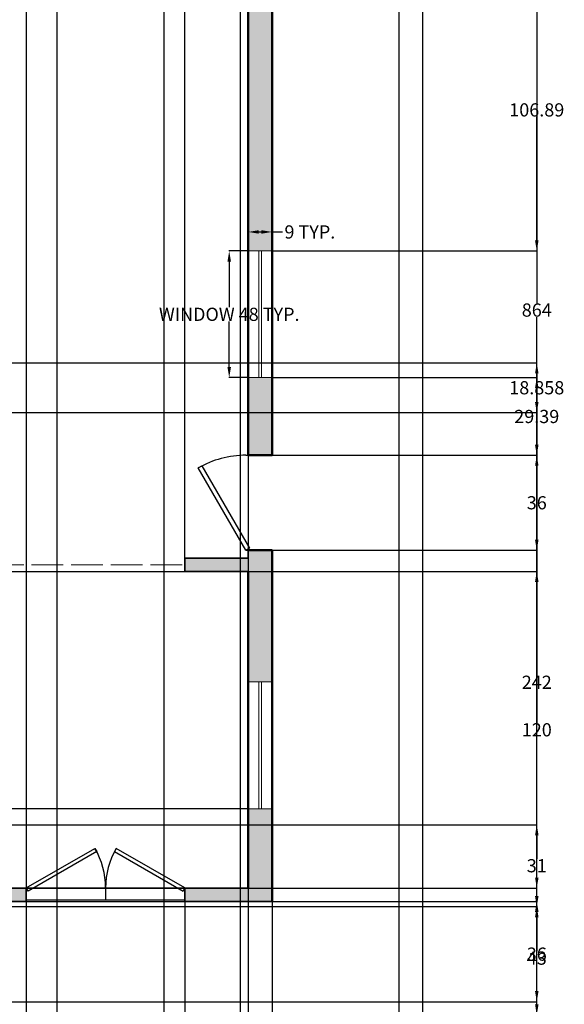
# Model space of a CAD drawing. Units: inches. Extents: x 882 to 1363, y 890 to 1847.
# Tile 6 of 9: x 1157 to 1363, y 1106 to 1479. Entities that reach past the tile are written whole.
import ezdxf

# ---------------------------------------------------------------- set-up
doc = ezdxf.new("R2010")
doc.units = ezdxf.units.IN
doc.header["$MEASUREMENT"] = 0
doc.linetypes.add('ACAD_ISO02W100', pattern=[15, 12, -3])
for name, color, linetype, lineweight in [('A-ANNO-DIMS', 2, 'Continuous', 18), ('A-WALL-OVHD', 7, 'ACAD_ISO02W100', 18), ('C-PROP', 7, 'Continuous', 25), ('doors', 3, 'Continuous', 25), ('inner wall', 50, 'Continuous', 35), ('outer wall', 40, 'Continuous', 50), ('windows', 226, 'Continuous', 18)]:
    doc.layers.add(name, color=color, linetype=linetype, lineweight=lineweight)
doc.layers.add('A-WALL-PATT', color=251, linetype='Continuous', lineweight=13, true_color=0x636466)
doc.styles.get("Standard").update_dxf_attribs({"font": 'arial.ttf'})
doc.dimstyles.get("Standard").update_dxf_attribs({"dimtxt": 5, "dimasz": 4, "dimexe": 0.18, "dimexo": 0.0625, "dimgap": 0.09, "dimtad": 0, "dimtih": 1, "dimtoh": 1, "dimdec": 1, "dimzin": 0, "dimdsep": 46, "dimlunit": 3, "dimtxsty": 'Standard', "dimcen": 0.09, "dimadec": 0, "dimazin": 0, "dimtfac": 1, "dimtdec": 1, "dimtofl": 0, "dimtmove": 0, "dimatfit": 3, "dimfxl": 1, "dimtolj": 1, "dimtzin": 0, "dimarcsym": 0})

# ---------------------------------------------------------------- blocks, each defined once
blk = doc.blocks.new('*U2')
for p, q in [((0, 0), (0, -6)), ((40, 0), (40, -6))]:
    blk.add_line(p, q)
blk.add_lwpolyline([(0, 0), (34.64, 20), (35.52, 18.48), (0.87, -1.52)], close=True)
blk.add_arc((0, 0), 40, 0, 30)
blk = doc.blocks.new('*U4')
for p, q in [((0, 0), (0, -6)), ((-40, 0), (-40, -6))]:
    blk.add_line(p, q)
blk.add_lwpolyline([(0, 0), (-34.64, 20), (-35.52, 18.48), (-0.88, -1.52)], close=True)
blk.add_arc((0, 0), 40, 150, 180)
blk = doc.blocks.new('WIN-48IN-9IN')
for p, q in [((4, 0), (4, 48)), ((5, 0), (5, 48))]:
    blk.add_line(p, q)
blk.add_lwpolyline([(0, 48), (9, 48), (9, 0), (0, 0)], close=True)
blk = doc.blocks.new('*D15')
at = {"layer": 'A-ANNO-DIMS', "color": 0, "lineweight": -2, "transparency": 16777216}
for p, q in [((1243.78, 1391.14), (1236.46, 1391.14)), ((1236.64, 1387.14), (1236.64, 1369.82)), ((1236.64, 1347.14), (1236.64, 1364.46)), ((1243.78, 1343.14), (1236.46, 1343.14))]:
    blk.add_line(p, q, dxfattribs=at)
at = {"layer": 'A-ANNO-DIMS', "color": 0, "transparency": 16777216}
for points in [[(1235.97, 1387.14), (1237.31, 1387.14), (1236.64, 1391.14)], [(1235.97, 1347.14), (1237.31, 1347.14), (1236.64, 1343.14)]]:
    blk.add_solid(points, dxfattribs=at)
at = {"layer": 'Defpoints', "color": 0, "transparency": 16777216}
for p in [(1236.64, 1391.14), (1243.84, 1391.14), (1243.84, 1343.14)]:
    blk.add_point(p, dxfattribs=at)
at = {"layer": 'A-ANNO-DIMS', "color": 0, "transparency": 16777216, "insert": (1236.64, 1367.14), "char_height": 5, "attachment_point": 5}
blk.add_mtext('\\A1;WINDOW 48 TYP.', dxfattribs=at)
blk = doc.blocks.new('*D16')
at = {"layer": 'A-ANNO-DIMS', "color": 0, "lineweight": -2, "transparency": 16777216}
for p, q in [((1243.84, 1391.2), (1243.84, 1398.52)), ((1247.84, 1398.34), (1248.84, 1398.34)), ((1252.84, 1391.2), (1252.84, 1398.52)), ((1252.84, 1398.34), (1256.84, 1398.34))]:
    blk.add_line(p, q, dxfattribs=at)
at = {"layer": 'A-ANNO-DIMS', "color": 0, "transparency": 16777216}
for points in [[(1247.84, 1399.01), (1247.84, 1397.67), (1243.84, 1398.34)], [(1248.84, 1399.01), (1248.84, 1397.67), (1252.84, 1398.34)]]:
    blk.add_solid(points, dxfattribs=at)
at = {"layer": 'Defpoints', "color": 0, "transparency": 16777216}
for p in [(1252.84, 1398.34), (1243.84, 1391.14), (1252.84, 1391.14)]:
    blk.add_point(p, dxfattribs=at)
at = {"layer": 'A-ANNO-DIMS', "color": 0, "transparency": 16777216, "insert": (1267.16, 1398.34), "char_height": 5, "attachment_point": 5}
blk.add_mtext('\\A1;9 TYP.', dxfattribs=at)
blk = doc.blocks.new('*D34')
at = {"layer": 'A-ANNO-DIMS', "color": 0, "lineweight": -2, "transparency": 16777216}
for p, q in [((1309.9, 1800.75), (1353.22, 1800.75)), ((1353.04, 1796.75), (1353.04, 1371.39)), ((1353.04, 940.75), (1353.04, 1366.11)), ((1309.9, 936.75), (1353.22, 936.75))]:
    blk.add_line(p, q, dxfattribs=at)
at = {"layer": 'A-ANNO-DIMS', "color": 0, "transparency": 16777216}
for points in [[(1352.38, 1796.75), (1353.71, 1796.75), (1353.04, 1800.75)], [(1352.38, 940.75), (1353.71, 940.75), (1353.04, 936.75)]]:
    blk.add_solid(points, dxfattribs=at)
at = {"layer": 'Defpoints', "color": 0, "transparency": 16777216}
for p in [(1309.84, 1800.75), (1353.04, 1800.75), (1309.84, 936.75)]:
    blk.add_point(p, dxfattribs=at)
at = {"layer": 'A-ANNO-DIMS', "color": 0, "transparency": 16777216, "insert": (1353.04, 1368.75), "char_height": 5, "attachment_point": 5}
blk.add_mtext('\\A1;864', dxfattribs=at)
blk = doc.blocks.new('*D42')
at = {"layer": 'A-ANNO-DIMS', "color": 0, "lineweight": -2, "transparency": 16777216}
for p, q in [((1159.84, 1710.69), (1159.84, 893.37)), ((1243.84, 1705.69), (1243.84, 893.37)), ((1163.84, 893.55), (1198.17, 893.55)), ((1239.84, 893.55), (1205.5, 893.55))]:
    blk.add_line(p, q, dxfattribs=at)
at = {"layer": 'A-ANNO-DIMS', "color": 0, "transparency": 16777216}
for points in [[(1163.84, 894.21), (1163.84, 892.88), (1159.84, 893.55)], [(1239.84, 894.21), (1239.84, 892.88), (1243.84, 893.55)]]:
    blk.add_solid(points, dxfattribs=at)
at = {"layer": 'Defpoints', "color": 0, "transparency": 16777216}
for p in [(1159.84, 1710.75), (1243.84, 1705.75), (1243.84, 893.55)]:
    blk.add_point(p, dxfattribs=at)
at = {"layer": 'A-ANNO-DIMS', "color": 0, "transparency": 16777216, "insert": (1201.84, 893.55), "char_height": 5, "attachment_point": 5}
blk.add_mtext('\\A1;84', dxfattribs=at)
blk = doc.blocks.new('*D49')
at = {"layer": 'A-ANNO-DIMS', "color": 0, "lineweight": -2, "transparency": 16777216}
for p, q in [((1211.84, 1562.69), (1211.84, 893.37)), ((1240.84, 1562.69), (1240.84, 893.37)), ((1215.84, 893.55), (1222.62, 893.55)), ((1236.84, 893.55), (1230.06, 893.55))]:
    blk.add_line(p, q, dxfattribs=at)
at = {"layer": 'A-ANNO-DIMS', "color": 0, "transparency": 16777216}
for points in [[(1215.84, 894.21), (1215.84, 892.88), (1211.84, 893.55)], [(1236.84, 894.21), (1236.84, 892.88), (1240.84, 893.55)]]:
    blk.add_solid(points, dxfattribs=at)
at = {"layer": 'Defpoints', "color": 0, "transparency": 16777216}
for p in [(1211.84, 1562.75), (1240.84, 1562.75), (1240.84, 893.55)]:
    blk.add_point(p, dxfattribs=at)
at = {"layer": 'A-ANNO-DIMS', "color": 0, "transparency": 16777216, "insert": (1226.34, 893.55), "char_height": 5, "attachment_point": 5}
blk.add_mtext('\\A1;29', dxfattribs=at)
blk = doc.blocks.new('*D53')
at = {"layer": 'A-ANNO-DIMS', "color": 0, "lineweight": -2, "transparency": 16777216}
for p, q in [((1142.86, 1767.69), (1142.86, 893.37)), ((1171.41, 1767.69), (1171.41, 893.37)), ((1138.86, 893.55), (1134.86, 893.55)), ((1175.41, 893.55), (1179.41, 893.55))]:
    blk.add_line(p, q, dxfattribs=at)
at = {"layer": 'A-ANNO-DIMS', "color": 0, "transparency": 16777216}
for points in [[(1138.86, 894.21), (1138.86, 892.88), (1142.86, 893.55)], [(1175.41, 894.21), (1175.41, 892.88), (1171.41, 893.55)]]:
    blk.add_solid(points, dxfattribs=at)
at = {"layer": 'Defpoints', "color": 0, "transparency": 16777216}
for p in [(1142.86, 1767.75), (1171.41, 1767.75), (1171.41, 893.55)]:
    blk.add_point(p, dxfattribs=at)
at = {"layer": 'A-ANNO-DIMS', "color": 0, "transparency": 16777216, "insert": (1157.14, 893.55), "char_height": 5, "attachment_point": 5}
blk.add_mtext('\\A1;28.554', dxfattribs=at)
blk = doc.blocks.new('*D62')
at = {"layer": 'A-ANNO-DIMS', "color": 0, "lineweight": -2, "transparency": 16777216}
for p, q in [((991.9, 1348.75), (1353.22, 1348.75)), ((1353.04, 1344.75), (1353.04, 1230.35)), ((1353.04, 1110.75), (1353.04, 1225.15)), ((991.9, 1106.75), (1353.22, 1106.75))]:
    blk.add_line(p, q, dxfattribs=at)
at = {"layer": 'A-ANNO-DIMS', "color": 0, "transparency": 16777216}
for points in [[(1352.38, 1344.75), (1353.71, 1344.75), (1353.04, 1348.75)], [(1352.38, 1110.75), (1353.71, 1110.75), (1353.04, 1106.75)]]:
    blk.add_solid(points, dxfattribs=at)
at = {"layer": 'Defpoints', "color": 0, "transparency": 16777216}
for p in [(991.84, 1348.75), (991.84, 1106.75), (1353.04, 1106.75)]:
    blk.add_point(p, dxfattribs=at)
at = {"layer": 'A-ANNO-DIMS', "color": 0, "transparency": 16777216, "insert": (1353.04, 1227.75), "char_height": 5, "attachment_point": 5}
blk.add_mtext('\\A1;242', dxfattribs=at)
blk = doc.blocks.new('*D64')
at = {"layer": 'A-ANNO-DIMS', "color": 0, "lineweight": -2, "transparency": 16777216}
for p, q in [((1117.84, 1269.69), (1117.84, 893.37)), ((1243.84, 1269.69), (1243.84, 893.37)), ((1121.84, 893.55), (1175.46, 893.55)), ((1239.84, 893.55), (1186.22, 893.55))]:
    blk.add_line(p, q, dxfattribs=at)
at = {"layer": 'A-ANNO-DIMS', "color": 0, "transparency": 16777216}
for points in [[(1121.84, 894.21), (1121.84, 892.88), (1117.84, 893.55)], [(1239.84, 894.21), (1239.84, 892.88), (1243.84, 893.55)]]:
    blk.add_solid(points, dxfattribs=at)
at = {"layer": 'Defpoints', "color": 0, "transparency": 16777216}
for p in [(1117.84, 1269.75), (1243.84, 1269.75), (1243.84, 893.55)]:
    blk.add_point(p, dxfattribs=at)
at = {"layer": 'A-ANNO-DIMS', "color": 0, "transparency": 16777216, "insert": (1180.84, 893.55), "char_height": 5, "attachment_point": 5}
blk.add_mtext('\\A1;126', dxfattribs=at)
blk = doc.blocks.new('*D65')
at = {"layer": 'A-ANNO-DIMS', "color": 0, "lineweight": -2, "transparency": 16777216}
for p, q in [((1117.9, 1269.75), (1353.22, 1269.75)), ((1353.04, 1265.75), (1353.04, 1212.39)), ((1353.04, 1153.75), (1353.04, 1207.11)), ((1117.9, 1149.75), (1353.22, 1149.75))]:
    blk.add_line(p, q, dxfattribs=at)
at = {"layer": 'A-ANNO-DIMS', "color": 0, "transparency": 16777216}
for points in [[(1352.38, 1265.75), (1353.71, 1265.75), (1353.04, 1269.75)], [(1352.38, 1153.75), (1353.71, 1153.75), (1353.04, 1149.75)]]:
    blk.add_solid(points, dxfattribs=at)
at = {"layer": 'Defpoints', "color": 0, "transparency": 16777216}
for p in [(1117.84, 1269.75), (1353.04, 1269.75), (1117.84, 1149.75)]:
    blk.add_point(p, dxfattribs=at)
at = {"layer": 'A-ANNO-DIMS', "color": 0, "transparency": 16777216, "insert": (1353.04, 1209.75), "char_height": 5, "attachment_point": 5}
blk.add_mtext('\\A1;120', dxfattribs=at)
blk = doc.blocks.new('*D66')
at = {"layer": 'A-ANNO-DIMS', "color": 0, "lineweight": -2, "transparency": 16777216}
for p, q in [((1159.84, 1144.69), (1159.84, 893.37)), ((1219.84, 1144.69), (1219.84, 893.37)), ((1163.84, 893.55), (1186.16, 893.55)), ((1215.84, 893.55), (1193.52, 893.55))]:
    blk.add_line(p, q, dxfattribs=at)
at = {"layer": 'A-ANNO-DIMS', "color": 0, "transparency": 16777216}
for points in [[(1163.84, 894.21), (1163.84, 892.88), (1159.84, 893.55)], [(1215.84, 894.21), (1215.84, 892.88), (1219.84, 893.55)]]:
    blk.add_solid(points, dxfattribs=at)
at = {"layer": 'Defpoints', "color": 0, "transparency": 16777216}
for p in [(1159.84, 1144.75), (1219.84, 1144.75), (1219.84, 893.55)]:
    blk.add_point(p, dxfattribs=at)
at = {"layer": 'A-ANNO-DIMS', "color": 0, "transparency": 16777216, "insert": (1189.84, 893.55), "char_height": 5, "attachment_point": 5}
blk.add_mtext('\\A1;60', dxfattribs=at)
blk = doc.blocks.new('*D67')
at = {"layer": 'A-ANNO-DIMS', "color": 0, "lineweight": -2, "transparency": 16777216}
for p, q in [((1252.9, 1313.75), (1353.22, 1313.75)), ((1353.04, 1309.75), (1353.04, 1298.39)), ((1353.04, 1281.75), (1353.04, 1293.1)), ((1252.9, 1277.75), (1353.22, 1277.75))]:
    blk.add_line(p, q, dxfattribs=at)
at = {"layer": 'A-ANNO-DIMS', "color": 0, "transparency": 16777216}
for points in [[(1352.38, 1309.75), (1353.71, 1309.75), (1353.04, 1313.75)], [(1352.38, 1281.75), (1353.71, 1281.75), (1353.04, 1277.75)]]:
    blk.add_solid(points, dxfattribs=at)
at = {"layer": 'Defpoints', "color": 0, "transparency": 16777216}
for p in [(1252.84, 1313.75), (1353.04, 1313.75), (1252.84, 1277.75)]:
    blk.add_point(p, dxfattribs=at)
at = {"layer": 'A-ANNO-DIMS', "color": 0, "transparency": 16777216, "insert": (1353.04, 1295.75), "char_height": 5, "attachment_point": 5}
blk.add_mtext('\\A1;36', dxfattribs=at)
blk = doc.blocks.new('*D69')
at = {"layer": 'A-ANNO-DIMS', "color": 0, "lineweight": -2, "transparency": 16777216}
for p, q in [((1027.9, 1173.75), (1353.22, 1173.75)), ((1353.04, 1169.75), (1353.04, 1160.89)), ((1353.04, 1146.75), (1353.04, 1155.6)), ((1027.9, 1142.75), (1353.22, 1142.75))]:
    blk.add_line(p, q, dxfattribs=at)
at = {"layer": 'A-ANNO-DIMS', "color": 0, "transparency": 16777216}
for points in [[(1352.38, 1169.75), (1353.71, 1169.75), (1353.04, 1173.75)], [(1352.38, 1146.75), (1353.71, 1146.75), (1353.04, 1142.75)]]:
    blk.add_solid(points, dxfattribs=at)
at = {"layer": 'Defpoints', "color": 0, "transparency": 16777216}
for p in [(1027.84, 1173.75), (1353.04, 1173.75), (1027.84, 1142.75)]:
    blk.add_point(p, dxfattribs=at)
at = {"layer": 'A-ANNO-DIMS', "color": 0, "transparency": 16777216, "insert": (1353.04, 1158.25), "char_height": 5, "attachment_point": 5}
blk.add_mtext('\\A1;31', dxfattribs=at)
blk = doc.blocks.new('*D70')
at = {"layer": 'A-ANNO-DIMS', "color": 0, "lineweight": -2, "transparency": 16777216}
for p, q in [((1027.9, 1142.75), (1353.22, 1142.75)), ((1353.04, 1138.75), (1353.04, 1127.39)), ((1353.04, 1110.75), (1353.04, 1122.1)), ((991.9, 1106.75), (1353.22, 1106.75))]:
    blk.add_line(p, q, dxfattribs=at)
at = {"layer": 'A-ANNO-DIMS', "color": 0, "transparency": 16777216}
for points in [[(1352.38, 1138.75), (1353.71, 1138.75), (1353.04, 1142.75)], [(1352.38, 1110.75), (1353.71, 1110.75), (1353.04, 1106.75)]]:
    blk.add_solid(points, dxfattribs=at)
at = {"layer": 'Defpoints', "color": 0, "transparency": 16777216}
for p in [(1027.84, 1142.75), (991.84, 1106.75), (1353.04, 1106.75)]:
    blk.add_point(p, dxfattribs=at)
at = {"layer": 'A-ANNO-DIMS', "color": 0, "transparency": 16777216, "insert": (1353.04, 1124.75), "char_height": 5, "attachment_point": 5}
blk.add_mtext('\\A1;36', dxfattribs=at)
blk = doc.blocks.new('*D71')
at = {"layer": 'A-ANNO-DIMS', "color": 0, "lineweight": -2, "transparency": 16777216}
for p, q in [((1243.78, 1179.86), (906.46, 1179.86)), ((906.64, 1175.86), (906.64, 1167.45)), ((906.64, 1153.75), (906.64, 1162.16)), ((1243.78, 1149.75), (906.46, 1149.75))]:
    blk.add_line(p, q, dxfattribs=at)
at = {"layer": 'A-ANNO-DIMS', "color": 0, "transparency": 16777216}
for points in [[(905.97, 1175.86), (907.3, 1175.86), (906.64, 1179.86)], [(905.97, 1153.75), (907.3, 1153.75), (906.64, 1149.75)]]:
    blk.add_solid(points, dxfattribs=at)
at = {"layer": 'Defpoints', "color": 0, "transparency": 16777216}
for p in [(906.64, 1179.86), (1243.84, 1179.86), (1243.84, 1149.75)]:
    blk.add_point(p, dxfattribs=at)
at = {"layer": 'A-ANNO-DIMS', "color": 0, "transparency": 16777216, "insert": (906.64, 1164.8), "char_height": 5, "attachment_point": 5}
blk.add_mtext('\\A1;30.107', dxfattribs=at)
blk = doc.blocks.new('*D77')
at = {"layer": 'A-ANNO-DIMS', "color": 0, "lineweight": -2, "transparency": 16777216}
for p, q in [((1117.9, 1144.75), (1353.22, 1144.75)), ((1353.04, 1140.75), (1353.04, 1125.89)), ((1353.04, 1105.75), (1353.04, 1120.6)), ((1117.9, 1101.75), (1353.22, 1101.75))]:
    blk.add_line(p, q, dxfattribs=at)
at = {"layer": 'A-ANNO-DIMS', "color": 0, "transparency": 16777216}
for points in [[(1352.38, 1140.75), (1353.71, 1140.75), (1353.04, 1144.75)], [(1352.38, 1105.75), (1353.71, 1105.75), (1353.04, 1101.75)]]:
    blk.add_solid(points, dxfattribs=at)
at = {"layer": 'Defpoints', "color": 0, "transparency": 16777216}
for p in [(1117.84, 1144.75), (1353.04, 1144.75), (1117.84, 1101.75)]:
    blk.add_point(p, dxfattribs=at)
at = {"layer": 'A-ANNO-DIMS', "color": 0, "transparency": 16777216, "insert": (1353.04, 1123.25), "char_height": 5, "attachment_point": 5}
blk.add_mtext('\\A1;43', dxfattribs=at)
blk = doc.blocks.new('*D78')
at = {"layer": 'A-ANNO-DIMS', "color": 0, "lineweight": -2, "transparency": 16777216}
for p, q in [((1146.84, 1274.81), (1146.84, 1844.13)), ((1150.84, 1843.95), (1179.69, 1843.95)), ((1215.84, 1843.95), (1186.99, 1843.95)), ((1219.84, 1274.81), (1219.84, 1844.13))]:
    blk.add_line(p, q, dxfattribs=at)
at = {"layer": 'A-ANNO-DIMS', "color": 0, "transparency": 16777216}
for points in [[(1150.84, 1844.62), (1150.84, 1843.29), (1146.84, 1843.95)], [(1215.84, 1844.62), (1215.84, 1843.29), (1219.84, 1843.95)]]:
    blk.add_solid(points, dxfattribs=at)
at = {"layer": 'Defpoints', "color": 0, "transparency": 16777216}
for p in [(1219.84, 1843.95), (1146.84, 1274.75), (1219.84, 1274.75)]:
    blk.add_point(p, dxfattribs=at)
at = {"layer": 'A-ANNO-DIMS', "color": 0, "transparency": 16777216, "insert": (1183.34, 1843.95), "char_height": 5, "attachment_point": 5}
blk.add_mtext('\\A1;73', dxfattribs=at)
blk = doc.blocks.new('*D80')
at = {"layer": 'A-ANNO-DIMS', "color": 0, "lineweight": -2, "transparency": 16777216}
for p, q in [((1252.9, 1498.03), (1353.22, 1498.03)), ((1353.04, 1494.03), (1353.04, 1447.23)), ((1353.04, 1395.14), (1353.04, 1441.94)), ((1252.9, 1391.14), (1353.22, 1391.14))]:
    blk.add_line(p, q, dxfattribs=at)
at = {"layer": 'A-ANNO-DIMS', "color": 0, "transparency": 16777216}
for points in [[(1352.38, 1494.03), (1353.71, 1494.03), (1353.04, 1498.03)], [(1352.38, 1395.14), (1353.71, 1395.14), (1353.04, 1391.14)]]:
    blk.add_solid(points, dxfattribs=at)
at = {"layer": 'Defpoints', "color": 0, "transparency": 16777216}
for p in [(1252.84, 1498.03), (1353.04, 1498.03), (1252.84, 1391.14)]:
    blk.add_point(p, dxfattribs=at)
at = {"layer": 'A-ANNO-DIMS', "color": 0, "transparency": 16777216, "insert": (1353.04, 1444.58), "char_height": 5, "attachment_point": 5}
blk.add_mtext('\\A1;106.89', dxfattribs=at)
blk = doc.blocks.new('*D81')
at = {"layer": 'A-ANNO-DIMS', "color": 0, "lineweight": -2, "transparency": 16777216}
for p, q in [((1252.9, 1343.14), (1353.22, 1343.14)), ((1353.04, 1339.14), (1353.04, 1331.09)), ((1353.04, 1317.75), (1353.04, 1325.8)), ((1252.9, 1313.75), (1353.22, 1313.75))]:
    blk.add_line(p, q, dxfattribs=at)
at = {"layer": 'A-ANNO-DIMS', "color": 0, "transparency": 16777216}
for points in [[(1352.38, 1339.14), (1353.71, 1339.14), (1353.04, 1343.14)], [(1352.38, 1317.75), (1353.71, 1317.75), (1353.04, 1313.75)]]:
    blk.add_solid(points, dxfattribs=at)
at = {"layer": 'Defpoints', "color": 0, "transparency": 16777216}
for p in [(1252.84, 1343.14), (1353.04, 1343.14), (1252.84, 1313.75)]:
    blk.add_point(p, dxfattribs=at)
at = {"layer": 'A-ANNO-DIMS', "color": 0, "transparency": 16777216, "insert": (1353.04, 1328.44), "char_height": 5, "attachment_point": 5}
blk.add_mtext('\\A1;29.39', dxfattribs=at)
blk = doc.blocks.new('*D82')
at = {"layer": 'A-ANNO-DIMS', "color": 0, "lineweight": -2, "transparency": 16777216}
for p, q in [((1219.84, 1144.69), (1219.84, 893.37)), ((1252.84, 1144.69), (1252.84, 893.37)), ((1223.84, 893.55), (1232.67, 893.55)), ((1248.84, 893.55), (1240.01, 893.55))]:
    blk.add_line(p, q, dxfattribs=at)
at = {"layer": 'A-ANNO-DIMS', "color": 0, "transparency": 16777216}
for points in [[(1223.84, 894.21), (1223.84, 892.88), (1219.84, 893.55)], [(1248.84, 894.21), (1248.84, 892.88), (1252.84, 893.55)]]:
    blk.add_solid(points, dxfattribs=at)
at = {"layer": 'Defpoints', "color": 0, "transparency": 16777216}
for p in [(1219.84, 1144.75), (1252.84, 1144.75), (1252.84, 893.55)]:
    blk.add_point(p, dxfattribs=at)
at = {"layer": 'A-ANNO-DIMS', "color": 0, "transparency": 16777216, "insert": (1236.34, 893.55), "char_height": 5, "attachment_point": 5}
blk.add_mtext('\\A1;33', dxfattribs=at)
blk = doc.blocks.new('*D88')
at = {"layer": 'A-ANNO-DIMS', "color": 0, "lineweight": -2, "transparency": 16777216}
for p, q in [((1128.84, 1567.69), (1128.84, 893.37)), ((1211.84, 1562.69), (1211.84, 893.37)), ((1132.84, 893.55), (1166.66, 893.55)), ((1207.84, 893.55), (1174.01, 893.55))]:
    blk.add_line(p, q, dxfattribs=at)
at = {"layer": 'A-ANNO-DIMS', "color": 0, "transparency": 16777216}
for points in [[(1132.84, 894.21), (1132.84, 892.88), (1128.84, 893.55)], [(1207.84, 894.21), (1207.84, 892.88), (1211.84, 893.55)]]:
    blk.add_solid(points, dxfattribs=at)
at = {"layer": 'Defpoints', "color": 0, "transparency": 16777216}
for p in [(1128.84, 1567.75), (1211.84, 1562.75), (1211.84, 893.55)]:
    blk.add_point(p, dxfattribs=at)
at = {"layer": 'A-ANNO-DIMS', "color": 0, "transparency": 16777216, "insert": (1170.34, 893.55), "char_height": 5, "attachment_point": 5}
blk.add_mtext('\\A1;83', dxfattribs=at)
blk = doc.blocks.new('*D94')
at = {"layer": 'A-ANNO-DIMS', "color": 0, "lineweight": -2, "transparency": 16777216}
for p, q in [((1128.9, 1348.75), (1353.22, 1348.75)), ((1353.04, 1344.75), (1353.04, 1341.96)), ((1353.04, 1333.89), (1353.04, 1336.68)), ((1049.35, 1329.89), (1353.22, 1329.89))]:
    blk.add_line(p, q, dxfattribs=at)
at = {"layer": 'A-ANNO-DIMS', "color": 0, "transparency": 16777216}
for points in [[(1352.38, 1344.75), (1353.71, 1344.75), (1353.04, 1348.75)], [(1352.38, 1333.89), (1353.71, 1333.89), (1353.04, 1329.89)]]:
    blk.add_solid(points, dxfattribs=at)
at = {"layer": 'Defpoints', "color": 0, "transparency": 16777216}
for p in [(1128.84, 1348.75), (1353.04, 1348.75), (1049.29, 1329.89)]:
    blk.add_point(p, dxfattribs=at)
at = {"layer": 'A-ANNO-DIMS', "color": 0, "transparency": 16777216, "insert": (1353.04, 1339.32), "char_height": 5, "attachment_point": 5}
blk.add_mtext('\\A1;18.858', dxfattribs=at)

msp = doc.modelspace()

# ---------------------------------------------------------------- hatches: boundary and pattern name
at = {"layer": 'A-WALL-PATT'}
h = msp.add_hatch(color=256, dxfattribs=at)
h.dxf.hatch_style = 1
h.paths.add_polyline_path([(1050.8388, 1481.7495), (1050.8388, 1478.7495), (1084.8388, 1478.7495), (1084.8388, 1473.7495), (991.8388, 1473.7495), (991.8388, 1361.0778), (982.8388, 1361.0778), (982.8388, 1556.1531), (991.8388, 1556.1531), (991.8388, 1478.7495), (1045.8388, 1478.7495), (1045.8388, 1481.7479), (1045.4161, 1481.7477), (1030.9055, 1506.8563), (1032.004, 1507.4911), (1046.5146, 1482.3825), (1045.4161, 1481.7477), (1045.8388, 1481.7479), (1045.8388, 1481.7495)])
h.paths.add_polyline_path([(1128.8388, 1478.7495), (1120.8388, 1478.7495), (1120.8388, 1473.7495), (1123.8388, 1473.7495), (1123.8388, 1353.7495), (991.8388, 1353.7495), (991.8388, 1361.0778), (982.8388, 1361.0778), (982.8388, 1337.3333), (991.8388, 1337.3333), (991.8388, 1348.7495), (1128.8388, 1348.7495)])
h.paths.add_polyline_path([(1118.8585, 1767.7495), (1048.8447, 1767.7495), (1048.8447, 1758.7495), (1064.8388, 1758.7495), (1069.8388, 1758.7495), (1118.8585, 1758.7495)])
h.paths.add_polyline_path([(1171.4129, 1767.7495), (1142.8585, 1767.7495), (1142.8585, 1758.7495), (1154.8388, 1758.7495), (1154.8388, 1710.7495), (1069.8388, 1710.7495), (1069.8388, 1713.7495), (1064.8388, 1713.7495), (1064.8388, 1705.7495), (1123.8388, 1705.7495), (1123.8388, 1567.7495), (1120.8388, 1567.7495), (1120.8388, 1562.7495), (1123.8388, 1562.7495), (1211.8388, 1562.7495), (1211.8388, 1567.7495), (1128.8388, 1567.7495), (1128.8388, 1705.7495), (1211.8388, 1705.7495), (1211.8388, 1710.7495), (1159.8388, 1710.7495), (1159.8388, 1758.7495), (1171.4129, 1758.7495)])
h.paths.add_polyline_path([(1252.8388, 1767.7495), (1195.4129, 1767.7495), (1195.4129, 1758.7495), (1243.8388, 1758.7495), (1243.8388, 1710.7495), (1240.8388, 1710.7495), (1240.8388, 1706.4648), (1240.8388, 1705.7495), (1243.8388, 1705.7495), (1243.8388, 1673.1735), (1252.8388, 1673.1735)])
h.paths.add_polyline_path([(1252.8388, 1625.1735), (1243.8388, 1625.1735), (1243.8388, 1567.7495), (1240.8388, 1567.7495), (1240.8388, 1562.7495), (1243.8388, 1562.7495), (1243.8388, 1546.029), (1252.8388, 1546.029)])
h.paths.add_polyline_path([(1252.8388, 1498.029), (1243.8388, 1498.029), (1243.8388, 1391.1399), (1252.8388, 1391.1399)])
h.paths.add_polyline_path([(1252.8388, 1179.8561), (1243.8388, 1179.8561), (1243.8388, 1149.7495), (1219.8388, 1149.7495), (1219.8388, 1145.3111), (1219.8388, 1144.7495), (1252.8388, 1144.7495)])
h.paths.add_polyline_path([(1252.8388, 1277.7495), (1243.8388, 1277.7495), (1243.8388, 1274.7495), (1219.8388, 1274.7495), (1219.8388, 1269.7495), (1243.8388, 1269.7495), (1243.8388, 1227.8561), (1252.8388, 1227.8561)])
h.paths.add_polyline_path([(1252.8388, 1343.1399), (1243.8388, 1343.1399), (1243.8388, 1313.7495), (1248.3388, 1313.7495), (1252.8388, 1313.7495)])
h.paths.add_polyline_path([(1146.8388, 1274.7495), (1112.8388, 1274.7495), (1112.8388, 1106.7495), (1106.7761, 1106.7495), (1106.7761, 1101.7495), (1117.8388, 1101.7495), (1117.8388, 1144.7495), (1159.8388, 1144.7495), (1159.8388, 1149.7495), (1117.8388, 1149.7495), (1117.8388, 1269.7495), (1146.8388, 1269.7495)])

# ---------------------------------------------------------------- linework, layer by layer
at = {"layer": 'A-WALL-OVHD'}
msp.add_line((1146.8388, 1272.2495), (1219.8388, 1272.2495), dxfattribs=at)
at = {"layer": 'C-PROP'}
for points in [[(949.8388, 1800.7495), (1309.8388, 1800.7495), (1309.8388, 936.7495), (949.8388, 936.7495)], [(958.8388, 1791.7495), (1300.8388, 1791.7495), (1300.8388, 945.7495), (958.8388, 945.7495)]]:
    msp.add_lwpolyline(points, close=True, dxfattribs=at)
at = {"layer": 'doors'}
msp.add_line((1159.8388, 1145.3111), (1219.8388, 1145.3111), dxfattribs=at)
at = {"layer": 'inner wall'}
for p, q in [((1243.8388, 1277.7495), (1243.8388, 1274.7495)), ((1219.8388, 1274.7495), (1219.8388, 1269.7495)), ((1219.8388, 1274.7495), (1243.8388, 1274.7495)), ((1219.8388, 1269.7495), (1243.8388, 1269.7495)), ((1117.8388, 1149.7495), (1159.8388, 1149.7495)), ((1159.8388, 1149.7495), (1159.8388, 1144.7495)), ((1219.8388, 1149.7495), (1219.8388, 1144.7495)), ((1219.8388, 1149.7495), (1243.8388, 1149.7495)), ((1117.8388, 1144.7495), (1159.8388, 1144.7495)), ((1219.8388, 1144.7495), (1252.8388, 1144.7495))]:
    msp.add_line(p, q, dxfattribs=at)
at = {"layer": 'outer wall'}
for p, q in [((1252.8388, 1767.7495), (1252.8388, 1313.7495)), ((1243.8388, 1562.7495), (1243.8388, 1313.7495)), ((1243.8388, 1313.7495), (1252.8388, 1313.7495)), ((1243.8388, 1277.7495), (1252.8388, 1277.7495)), ((1252.8388, 1277.7495), (1252.8388, 1144.7495)), ((1243.8388, 1269.7495), (1243.8388, 1149.7495))]:
    msp.add_line(p, q, dxfattribs=at)

# ---------------------------------------------------------------- block references
at = {"layer": 'doors', "xscale": 0.9, "yscale": 0.9, "zscale": 0.9, "rotation": 90}
msp.add_blockref('*U2', (1242.9388, 1277.7495), dxfattribs=at)
at = {"layer": 'doors', "xscale": 0.75, "yscale": 0.75, "zscale": 0.75}
for name, p in [('*U2', (1159.8388, 1149.8111)), ('*U4', (1219.8388, 1149.8111))]:
    msp.add_blockref(name, p, dxfattribs=at)
at = {"layer": 'windows'}
for p in [(1243.839, 1343.1401), (1243.839, 1179.8563)]:
    msp.add_blockref('WIN-48IN-9IN', p, dxfattribs=at)

# ---------------------------------------------------------------- dimensions: what is measured, and where the dimension line sits
at = {"layer": 'A-ANNO-DIMS'}
for base, p1, p2, override, picture, middle in [((1219.8388, 1843.953), (1146.8388, 1274.7495), (1219.8388, 1274.7495), {"dimdec": 0, "dimlfac": 1, "dimrnd": 0, "dimzin": 0, "dimdsep": 46, "dimlunit": 2}, '*D78', (1183.3388, 1843.953)), ((1171.4129, 893.546), (1142.8585, 1767.7495), (1171.4129, 1767.7495), {"dimdec": 3, "dimlfac": 1, "dimrnd": 0, "dimzin": 0, "dimdsep": 46, "dimlunit": 2}, '*D53', (1157.1357, 893.546)), ((1243.8388, 893.546), (1159.8388, 1710.7495), (1243.8388, 1705.7495), {"dimdec": 0, "dimlfac": 1, "dimrnd": 0, "dimzin": 0, "dimdsep": 46, "dimlunit": 2}, '*D42', (1201.8388, 893.546)), ((1211.8388, 893.546), (1128.8388, 1567.7495), (1211.8388, 1562.7495), {"dimdec": 0, "dimlfac": 1, "dimrnd": 0, "dimzin": 0, "dimdsep": 46, "dimlunit": 2}, '*D88', (1170.3388, 893.546)), ((1240.8388, 893.546), (1211.8388, 1562.7495), (1240.8388, 1562.7495), {"dimdec": 0, "dimlfac": 1, "dimrnd": 0, "dimzin": 0, "dimdsep": 46, "dimlunit": 2}, '*D49', (1226.3388, 893.546)), ((1243.8388, 893.546), (1117.8388, 1269.7495), (1243.8388, 1269.7495), {"dimdec": 0, "dimlfac": 1, "dimrnd": 0, "dimzin": 0, "dimdsep": 46, "dimlunit": 2}, '*D64', (1180.8388, 893.546)), ((1219.8388, 893.546), (1159.8388, 1144.7495), (1219.8388, 1144.7495), {"dimdec": 0, "dimlfac": 1, "dimrnd": 0, "dimzin": 0, "dimdsep": 46, "dimlunit": 2}, '*D66', (1189.8388, 893.546)), ((1252.8388, 893.546), (1219.8388, 1144.7495), (1252.8388, 1144.7495), {"dimdec": 0, "dimlfac": 1, "dimrnd": 0, "dimzin": 0, "dimdsep": 46, "dimlunit": 2}, '*D82', (1236.3388, 893.546))]:
    dim = msp.add_linear_dim(base=base, p1=p1, p2=p2, dimstyle='Standard', override=override, dxfattribs=at)
    dim.commit()
    dim.dimension.update_dxf_attribs({"geometry": picture, "text_midpoint": middle})
for base, p1, p2, override, picture, middle in [((1353.0423, 1800.7495), (1309.8388, 936.7495), (1309.8388, 1800.7495), {"dimdec": 0, "dimlfac": 1, "dimrnd": 0, "dimzin": 0, "dimdsep": 46, "dimlunit": 2}, '*D34', (1353.0423, 1368.7495)), ((1353.0423, 1498.029), (1252.8388, 1391.1399), (1252.8388, 1498.029), {"dimdec": 2, "dimlfac": 1, "dimrnd": 0, "dimzin": 0, "dimdsep": 46, "dimlunit": 2}, '*D80', (1353.0423, 1444.5844)), ((1353.0423, 1106.7495), (991.8388, 1348.7495), (991.8388, 1106.7495), {"dimdec": 0, "dimlfac": 1, "dimrnd": 0, "dimzin": 0, "dimdsep": 46, "dimlunit": 2}, '*D62', (1353.0423, 1227.7495)), ((1353.0423, 1348.7495), (1049.2874, 1329.8919), (1128.8388, 1348.7495), {"dimdec": 3, "dimlfac": 1, "dimrnd": 0, "dimzin": 0, "dimdsep": 46, "dimlunit": 2}, '*D94', (1353.0423, 1339.3207)), ((1353.0423, 1343.1399), (1252.8388, 1313.7495), (1252.8388, 1343.1399), {"dimdec": 2, "dimlfac": 1, "dimrnd": 0, "dimzin": 0, "dimdsep": 46, "dimlunit": 2}, '*D81', (1353.0423, 1328.4447)), ((1353.0423, 1313.7495), (1252.8388, 1277.7495), (1252.8388, 1313.7495), {"dimdec": 0, "dimlfac": 1, "dimrnd": 0, "dimzin": 0, "dimdsep": 46, "dimlunit": 2}, '*D67', (1353.0423, 1295.7495)), ((1353.0423, 1269.7495), (1117.8388, 1149.7495), (1117.8388, 1269.7495), {"dimdec": 0, "dimlfac": 1, "dimrnd": 0, "dimzin": 0, "dimdsep": 46, "dimlunit": 2}, '*D65', (1353.0423, 1209.7495)), ((906.6353, 1179.8561), (1243.8388, 1149.7495), (1243.8388, 1179.8561), {"dimdec": 3, "dimlfac": 1, "dimrnd": 0, "dimzin": 0, "dimdsep": 46, "dimlunit": 2}, '*D71', (906.6353, 1164.8028)), ((1353.0423, 1173.7495), (1027.8388, 1142.7495), (1027.8388, 1173.7495), {"dimdec": 0, "dimlfac": 1, "dimrnd": 0, "dimzin": 0, "dimdsep": 46, "dimlunit": 2}, '*D69', (1353.0423, 1158.2495)), ((1353.0423, 1106.7495), (1027.8388, 1142.7495), (991.8388, 1106.7495), {"dimdec": 0, "dimlfac": 1, "dimrnd": 0, "dimzin": 0, "dimdsep": 46, "dimlunit": 2}, '*D70', (1353.0423, 1124.7495)), ((1353.0423, 1144.7495), (1117.8388, 1101.7495), (1117.8388, 1144.7495), {"dimdec": 0, "dimlfac": 1, "dimrnd": 0, "dimzin": 0, "dimdsep": 46, "dimlunit": 2}, '*D77', (1353.0423, 1123.2495))]:
    dim = msp.add_linear_dim(base=base, p1=p1, p2=p2, angle=90, dimstyle='Standard', override=override, dxfattribs=at)
    dim.commit()
    dim.dimension.update_dxf_attribs({"geometry": picture, "text_midpoint": middle})
dim = msp.add_linear_dim(base=(1252.8388, 1398.3399), p1=(1243.8388, 1391.1399), p2=(1252.8388, 1391.1399), text='<> TYP.', dimstyle='Standard', override={"dimdec": 0, "dimlfac": 1, "dimrnd": 0, "dimzin": 0, "dimdsep": 46, "dimlunit": 2}, dxfattribs=at)
dim.commit()
dim.dimension.update_dxf_attribs({"geometry": '*D16', "text_midpoint": (1267.1556, 1398.3399)})
dim = msp.add_linear_dim(base=(1236.6388, 1391.1399), p1=(1243.8388, 1343.1399), p2=(1243.8388, 1391.1399), angle=90, text='WINDOW <> TYP.', dimstyle='Standard', override={"dimdec": 0, "dimlfac": 1, "dimrnd": 0, "dimzin": 0, "dimdsep": 46, "dimlunit": 2}, dxfattribs=at)
dim.commit()
dim.dimension.update_dxf_attribs({"geometry": '*D15', "text_midpoint": (1236.6388, 1367.1399)})

doc.saveas('drawing.dxf')
